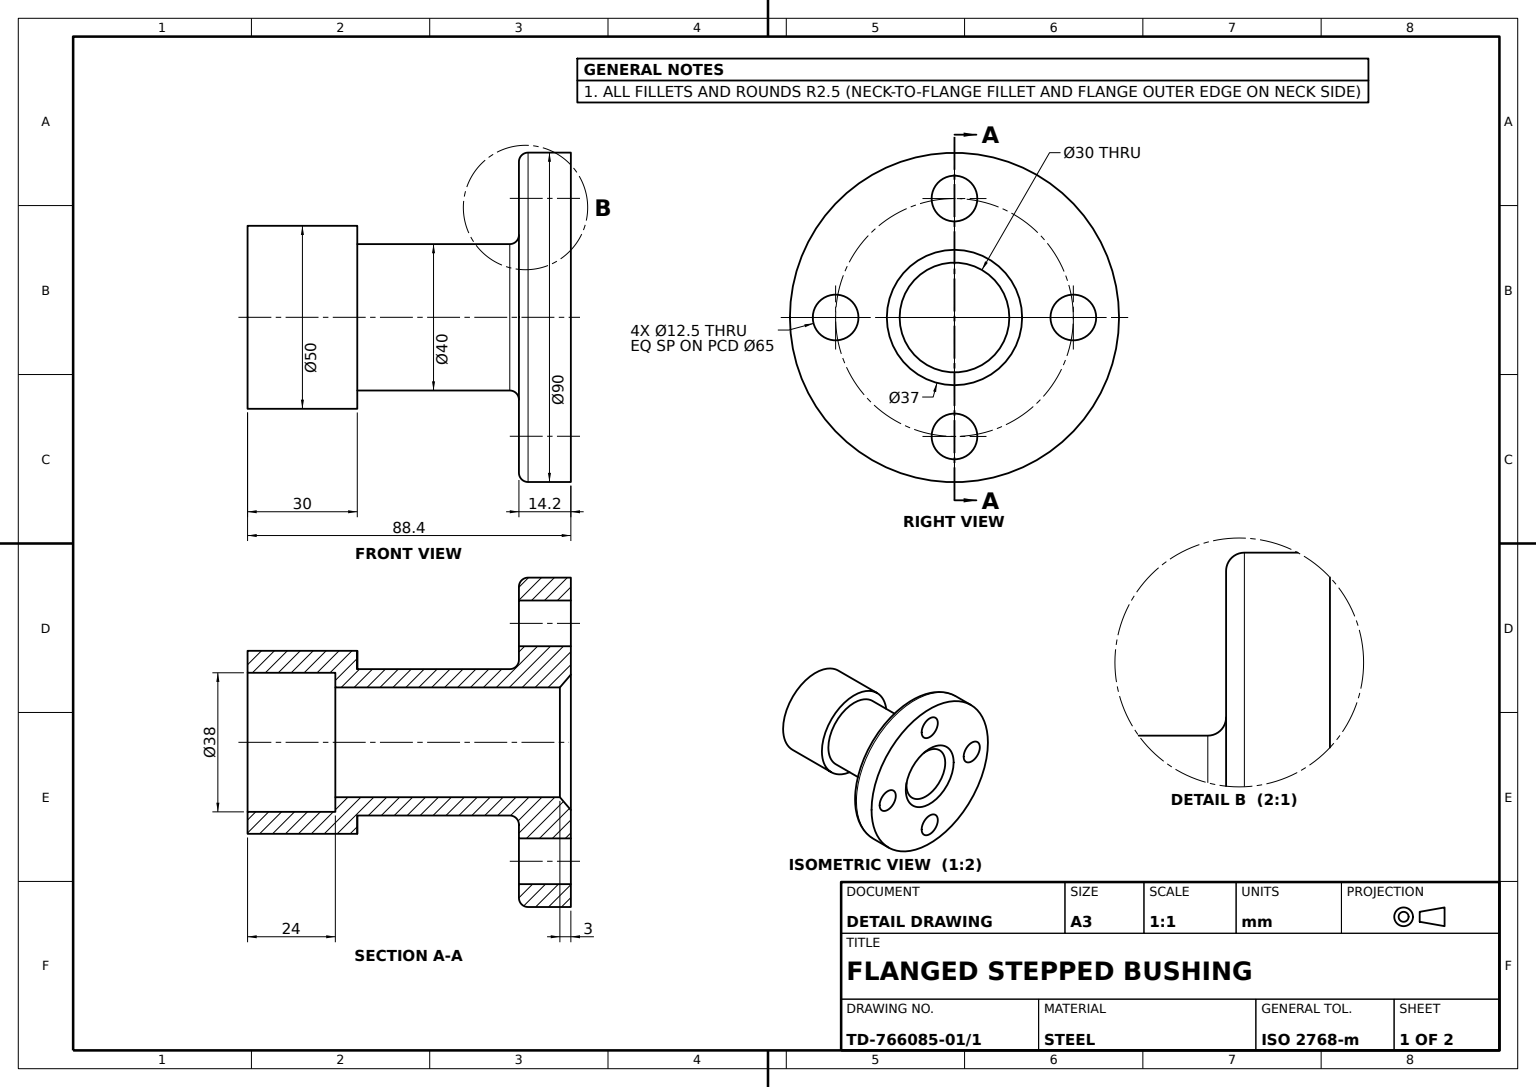
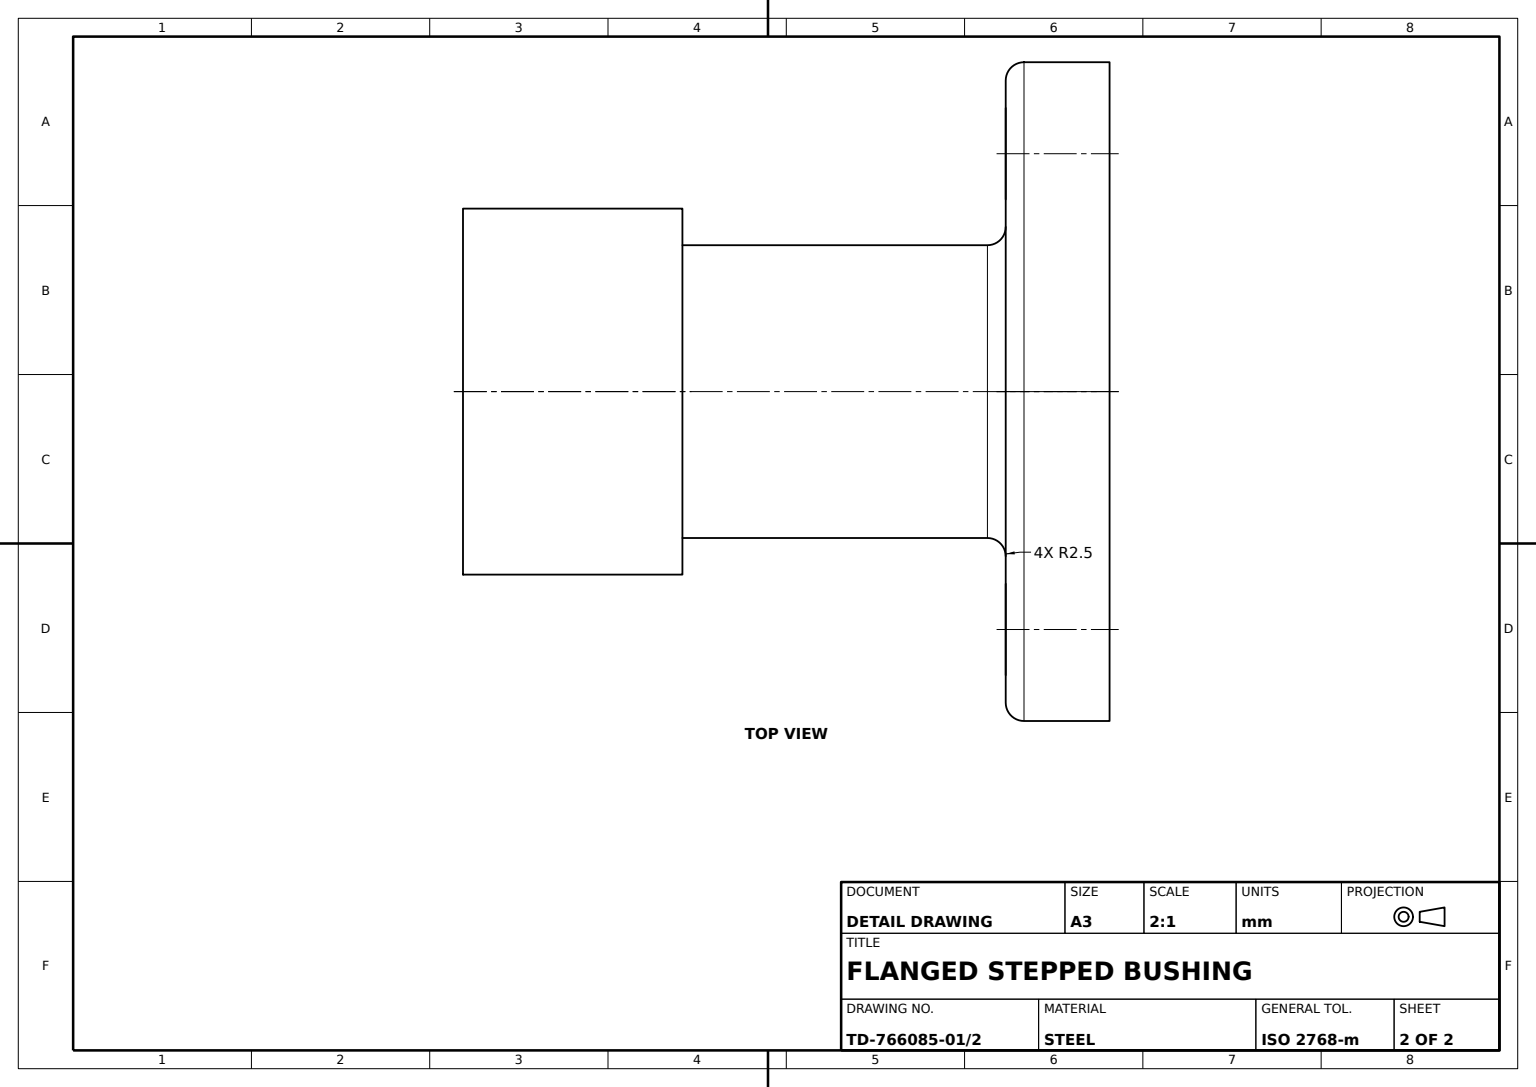
from build123d import *

# Parameters (mm, degrees)
FLANGE_PROFILE_SKETCH_R       = 45
FLANGE_PROFILE_SKETCH_R_2     = 15
FLANGE_90_DEPTH               = 14.2
FLANGE_HOLES_SKETCH_R         = 6.25
FLANGE_HOLES_4X_12_5_DEPTH    = 66.204601065
FLANGE_CHAMFER_SIZE           = 3
FLANGE_CHAMFER_SIZE2          = 3.5
NECK_PROFILE_SKETCH_R         = 20
NECK_PROFILE_SKETCH_R_2       = 15
NECK_40_DEPTH                 = 44.2
FLANGE_EDGE_FILLET_R2_5_R     = 2.5
COLLAR_PROFILE_SKETCH_R       = 25
COLLAR_PROFILE_SKETCH_R_2     = 15
COLLAR_50_DEPTH               = 6
END_SLEEVE_PROFILE_SKETCH_R   = 25
END_SLEEVE_PROFILE_SKETCH_R_2 = 19
END_SLEEVE_50_BORE_38_DEPTH   = 24
NECK_ROOT_FILLET_R2_5_R       = 2.5


with BuildPart() as part:
    # Flange Profile Sketch → Flange Ø90 (new body)
    with BuildSketch(Plane.XY):
        Circle(FLANGE_PROFILE_SKETCH_R)
        Circle(FLANGE_PROFILE_SKETCH_R_2, mode=Mode.SUBTRACT)
    extrude(amount=FLANGE_90_DEPTH)

    # Flange Holes Sketch → Flange Holes 4xØ12.5 (cut, through all)
    with BuildSketch(Plane(origin=(0, 0, 0), x_dir=(-1, 0, 0), z_dir=(0, 0, -1))):
        with Locations((-32.5, 0)):
            Circle(FLANGE_HOLES_SKETCH_R)
        with Locations((32.5, 0)):
            Circle(FLANGE_HOLES_SKETCH_R)
        with Locations((0, -32.5)):
            Circle(FLANGE_HOLES_SKETCH_R)
        with Locations((0, 32.5)):
            Circle(FLANGE_HOLES_SKETCH_R)
    extrude(amount=-FLANGE_HOLES_4X_12_5_DEPTH, mode=Mode.SUBTRACT)

    # Flange Chamfer
    flange_chamfer_edges = [part.edges().sort_by_distance(p)[0] for p in [
        (-15, 0, 0),
    ]]
    flange_chamfer_side = [part.faces().sort_by_distance(p)[0] for p in [
        (-15, 0, 7.1),
    ]]
    chamfer(flange_chamfer_edges, length=FLANGE_CHAMFER_SIZE, length2=FLANGE_CHAMFER_SIZE2, reference=flange_chamfer_side[0])

    # Neck Profile Sketch → Neck Ø40 (add)
    with BuildSketch(Plane.XY.offset(14.2)):
        Circle(NECK_PROFILE_SKETCH_R)
        Circle(NECK_PROFILE_SKETCH_R_2, mode=Mode.SUBTRACT)
    extrude(amount=NECK_40_DEPTH)

    # Flange Edge Fillet R2.5
    flange_edge_fillet_r2_5_edges = [part.edges().sort_by_distance(p)[0] for p in [
        (-45, 0, 14.2),
    ]]
    fillet(flange_edge_fillet_r2_5_edges, radius=FLANGE_EDGE_FILLET_R2_5_R)

    # Collar Profile Sketch → Collar Ø50 (add)
    with BuildSketch(Plane.XY.offset(58.4)):
        Circle(COLLAR_PROFILE_SKETCH_R)
        Circle(COLLAR_PROFILE_SKETCH_R_2, mode=Mode.SUBTRACT)
    extrude(amount=COLLAR_50_DEPTH)

    # End Sleeve Profile Sketch → End Sleeve Ø50 Bore Ø38 (add)
    with BuildSketch(Plane.XY.offset(64.4)):
        Circle(END_SLEEVE_PROFILE_SKETCH_R)
        Circle(END_SLEEVE_PROFILE_SKETCH_R_2, mode=Mode.SUBTRACT)
    extrude(amount=END_SLEEVE_50_BORE_38_DEPTH)

    # Neck Root Fillet R2.5
    neck_root_fillet_r2_5_edges = [part.edges().sort_by_distance(p)[0] for p in [
        (-20, 0, 14.2),
    ]]
    fillet(neck_root_fillet_r2_5_edges, radius=NECK_ROOT_FILLET_R2_5_R)


solid = part.part
